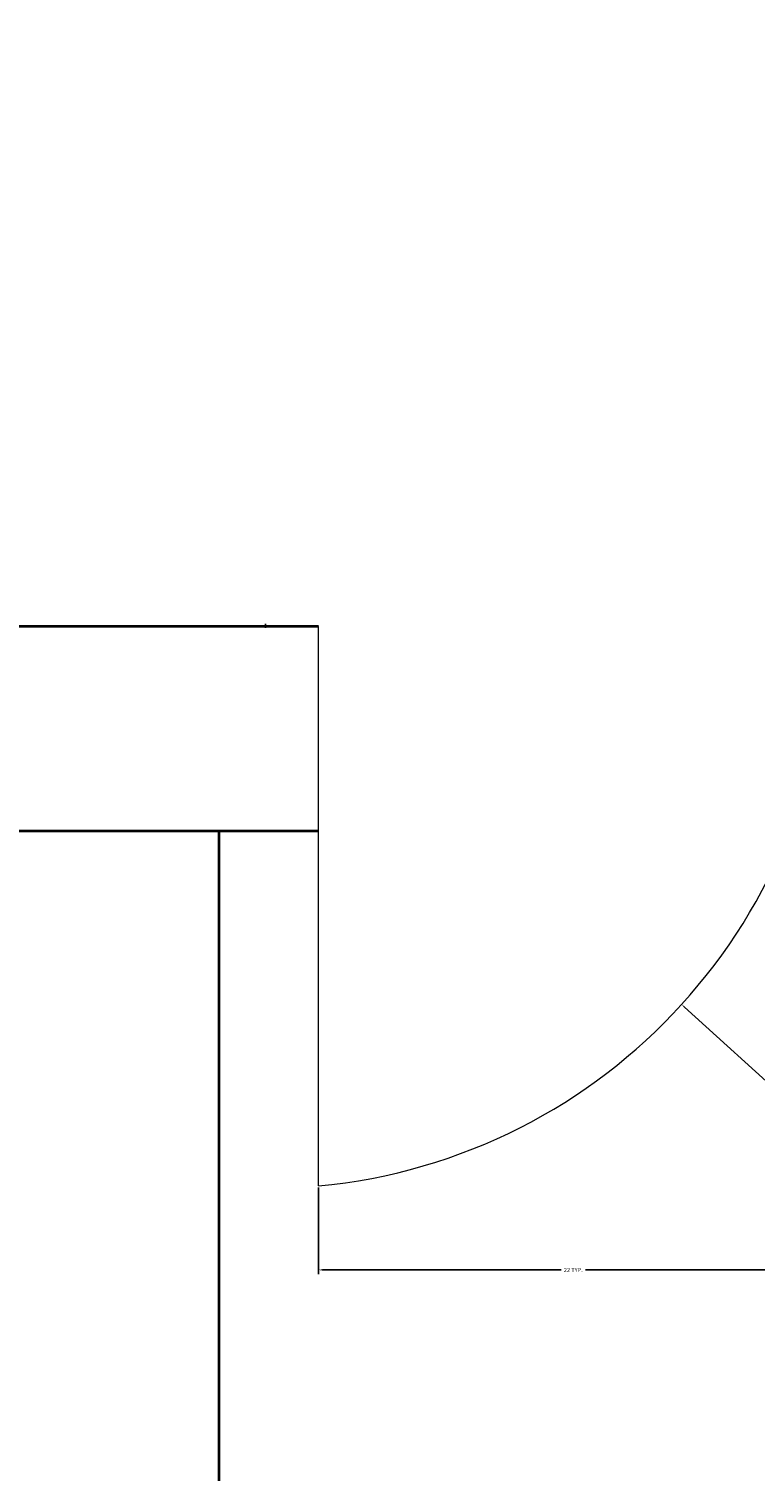
# Model space of a CAD drawing. Units: feet. Extents: x 5816 to 6644, y 25475 to 26788.
# Tile 19 of 23: x 6115 to 6147, y 26530 to 26594. Entities that reach past the tile are written whole.
import ezdxf

# ---------------------------------------------------------------- set-up
doc = ezdxf.new("R2010")
doc.units = ezdxf.units.FT
for name, color, linetype, lineweight in [('A-ANNO-DIMS', 2, 'Continuous', 13), ('A-DOOR', 3, 'Continuous', 18), ('A-WALL', 7, 'Continuous', 35)]:
    doc.layers.add(name, color=color, linetype=linetype, lineweight=lineweight)
doc.styles.get("Standard").update_dxf_attribs({"font": 'arial.ttf'})
doc.dimstyles.get("Standard").update_dxf_attribs({"dimtxt": 0.18, "dimasz": 0.18, "dimexe": 0.18, "dimexo": 0.0625, "dimgap": 0.09, "dimtad": 0, "dimtih": 1, "dimtoh": 1, "dimdec": 4, "dimzin": 0, "dimdsep": 46, "dimtxsty": 'Standard', "dimcen": 0.09, "dimadec": 0, "dimazin": 0, "dimtfac": 1, "dimtdec": 4, "dimtofl": 0, "dimtmove": 0, "dimatfit": 3, "dimfxl": 1, "dimtolj": 1, "dimtzin": 0, "dimarcsym": 0})

# ---------------------------------------------------------------- blocks, each defined once
blk = doc.blocks.new('DOOR-BATH-ENSUITE')
blk.add_line((0, -24.59), (0, 0))
blk.add_arc((-2.33, 0.023), 24.723, 275.40734, 0)
blk = doc.blocks.new('*D34')
at = {"layer": 'A-ANNO-DIMS', "color": 0, "lineweight": -2, "transparency": 16777216}
for p, q in [((6127.688, 26542.932), (6127.688, 26539.123)), ((6150.081, 26542.932), (6150.081, 26539.123)), ((6127.868, 26539.303), (6138.355, 26539.303)), ((6149.901, 26539.303), (6139.414, 26539.303))]:
    blk.add_line(p, q, dxfattribs=at)
at = {"layer": 'A-ANNO-DIMS', "color": 0, "transparency": 16777216}
for points in [[(6127.868, 26539.333), (6127.868, 26539.273), (6127.688, 26539.303)], [(6149.901, 26539.333), (6149.901, 26539.273), (6150.081, 26539.303)]]:
    blk.add_solid(points, dxfattribs=at)
at = {"layer": 'Defpoints', "color": 0, "transparency": 16777216}
for p in [(6127.688, 26542.995), (6150.081, 26542.995), (6150.081, 26539.303)]:
    blk.add_point(p, dxfattribs=at)
at = {"layer": 'A-ANNO-DIMS', "color": 0, "transparency": 16777216, "insert": (6138.884, 26539.303), "char_height": 0.18, "attachment_point": 5}
blk.add_mtext('\\A1;22 TYP.', dxfattribs=at)
blk = doc.blocks.new('*D60')
at = {"layer": 'A-ANNO-DIMS', "color": 0, "lineweight": -2, "transparency": 16777216}
for p, q in [((6106.978, 26094.399), (6106.978, 26787.915)), ((6107.158, 26787.735), (6224.932, 26787.735)), ((6343.496, 26787.735), (6225.722, 26787.735)), ((6343.676, 26094.399), (6343.676, 26787.915))]:
    blk.add_line(p, q, dxfattribs=at)
at = {"layer": 'A-ANNO-DIMS', "color": 0, "transparency": 16777216}
for points in [[(6107.158, 26787.765), (6107.158, 26787.705), (6106.978, 26787.735)], [(6343.496, 26787.765), (6343.496, 26787.705), (6343.676, 26787.735)]]:
    blk.add_solid(points, dxfattribs=at)
at = {"layer": 'Defpoints', "color": 0, "transparency": 16777216}
for p in [(6343.676, 26787.735), (6106.978, 26094.337), (6343.676, 26094.337)]:
    blk.add_point(p, dxfattribs=at)
at = {"layer": 'A-ANNO-DIMS', "color": 0, "transparency": 16777216, "insert": (6225.327, 26787.735), "char_height": 0.18, "attachment_point": 5}
blk.add_mtext('\\A1;236.7', dxfattribs=at)
blk = doc.blocks.new('*D80')
at = {"layer": 'A-ANNO-DIMS', "color": 0, "lineweight": -2, "transparency": 16777216}
for p, q in [((6125.268, 26567.608), (6125.448, 26567.608)), ((6125.358, 26567.518), (6125.358, 26567.698)), ((6154.617, 26540.987), (6143.778, 26550.849)), ((6154.797, 26540.987), (6154.617, 26540.987))]:
    blk.add_line(p, q, dxfattribs=at)
at = {"layer": 'A-ANNO-DIMS', "color": 0, "transparency": 16777216}
blk.add_solid([(6143.798, 26550.871), (6143.758, 26550.827), (6143.645, 26550.97)], dxfattribs=at)
at = {"layer": 'Defpoints', "color": 0, "transparency": 16777216}
for p in [(6125.358, 26567.608), (6143.645, 26550.97)]:
    blk.add_point(p, dxfattribs=at)
at = {"layer": 'A-ANNO-DIMS', "color": 0, "transparency": 16777216, "insert": (6155.544, 26540.987), "char_height": 0.18, "attachment_point": 5}
blk.add_mtext('\\A1;4X R24.723', dxfattribs=at)

msp = doc.modelspace()

# ---------------------------------------------------------------- linework, layer by layer
at = {"layer": 'A-WALL'}
for p, q in [((6127.6877, 26567.5846), (6103.9699, 26567.5846)), ((6127.6877, 26558.5846), (6103.9699, 26558.5846)), ((6123.3119, 26558.5846), (6123.3119, 26507.5846)), ((6127.6877, 26558.5846), (6123.3119, 26558.5846))]:
    msp.add_line(p, q, dxfattribs=at)

# ---------------------------------------------------------------- block references
at = {"layer": 'A-DOOR'}
msp.add_blockref('DOOR-BATH-ENSUITE', (6127.6877, 26567.5846), dxfattribs=at)

# ---------------------------------------------------------------- dimensions: what is measured, and where the dimension line sits
at = {"layer": 'A-ANNO-DIMS'}
dim = msp.add_linear_dim(base=(6343.6763, 26787.7346), p1=(6106.9781, 26094.3368), p2=(6343.6763, 26094.3368), dimstyle='Standard', override={"dimdec": 1, "dimlfac": 1, "dimrnd": 0, "dimzin": 0, "dimdsep": 46, "dimlunit": 2}, dxfattribs=at)
dim.commit()
dim.dimension.update_dxf_attribs({"geometry": '*D60', "text_midpoint": (6225.3272, 26787.7346)})
dim = msp.add_radius_dim(center=(6125.3579, 26567.608), mpoint=(6143.645, 26550.97), text='4X <>', dimstyle='Standard', override={"dimdec": 3, "dimlfac": 1, "dimrnd": 0, "dimzin": 0, "dimdsep": 46, "dimlunit": 2}, dxfattribs=at)
dim.commit()
dim.dimension.update_dxf_attribs({"geometry": '*D80', "text_midpoint": (6155.544, 26540.9872), "dimtype": 164})
dim = msp.add_linear_dim(base=(6150.0811, 26539.3028), p1=(6127.6877, 26542.9948), p2=(6150.0811, 26542.9948), text='<> TYP.', dimstyle='Standard', override={"dimdec": 0, "dimlfac": 1, "dimrnd": 0, "dimzin": 0, "dimdsep": 46, "dimlunit": 2}, dxfattribs=at)
dim.commit()
dim.dimension.update_dxf_attribs({"geometry": '*D34', "text_midpoint": (6138.8844, 26539.3028)})

doc.saveas('drawing.dxf')
